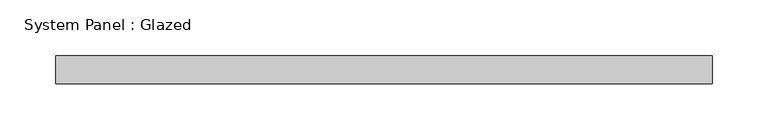
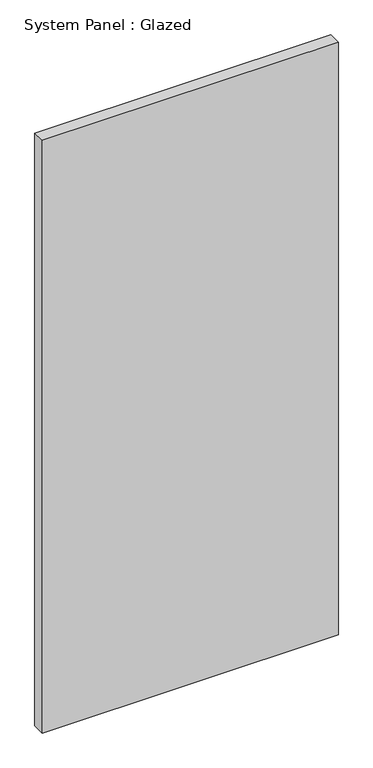
"""IFC4 building model written with IfcOpenShell, lengths in millimetres: plate geometry, System Panel : Glazed."""

from ifc_helpers import new_model, si_unit, origin, origin_with_axes, place, context, project, spatial, polyline, outline, extrude, source, transform, mapped, element, save


def system_panel_glazed_947315be(model_context):
    return source(origin(), model_context, "Body", "SweptSolid", [
        extrude(outline(polyline([(295.275, 19.05), (-295.275, 19.05), (-295.275, 44.45), (295.275, 44.45), (295.275, 19.05)])), origin_with_axes(), (0.0, 0.0, 1.0), 1248.9446538),
    ])


if __name__ == "__main__":
    model = new_model("IFC4")
    model_context = context("Model", 3, world=origin())
    ifc_project = project(units=[si_unit("LENGTHUNIT", "METRE", prefix="MILLI")], contexts=[model_context])
    site = spatial("IfcSite", under=ifc_project)
    building = spatial("IfcBuilding", under=site)
    placement = place(None, origin())
    system_panel_glazed_shape = system_panel_glazed_947315be(model_context)
    element("IfcPlate", 1, ObjectType="System Panel : Glazed", at=placement, inside=building, context=model_context, shape_type="MappedRepresentation", body=[
        mapped(system_panel_glazed_shape, transform((0.0, 0.0, 0.0), x_axis=(1.0, 0.0, 0.0), y_axis=(0.0, 1.0, 0.0), z_axis=(0.0, 0.0, 1.0))),
    ])
    save(model, "model.ifc")

# Revit data of these elements
# Type "System Panel : Glazed"
#   Construction Type Id = "GSP4R"
#   Analytic Construction = "1/8 in Pilkington single glazing"
#   Visual Light Transmittance = 0.9
#   Solar Heat Gain Coefficient = 0.86
#   Heat Transfer Coefficient (U) = 1.18115 BTU/(h·ft²·°F)
#   Define Thermal Properties by = 1
# Element 1 (IfcPlate, "System Panel : Glazed")
#   Materials on its faces: "Glass"
# Materials
#   "Glass": class "Glass", colour RGB 0 128 192, transparency 0.75, Description = "Soda Lime Glass", Cost = 0
